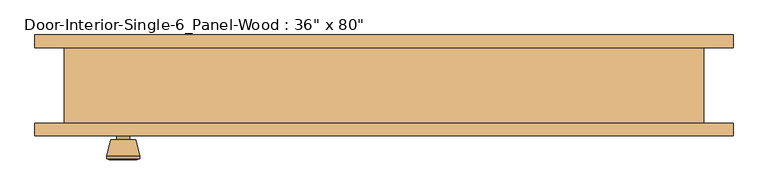
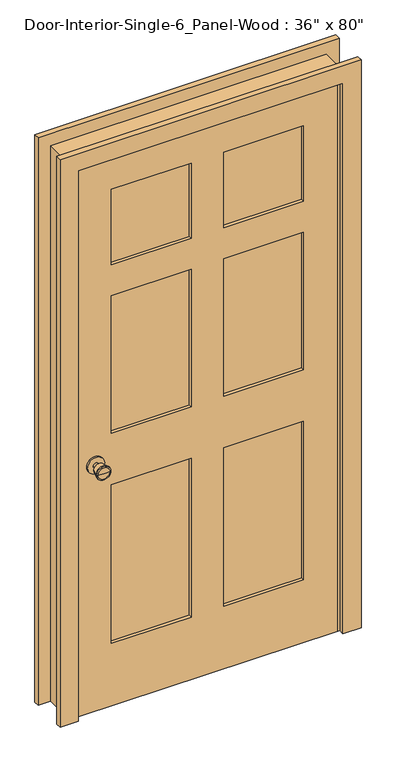
"""IFC4 building model written with IfcOpenShell, lengths in millimetres: door geometry."""

from ifc_helpers import new_model, si_unit, point, frame, frame_2d, origin, place, context, project, spatial, polyline, circle_curve, trimmed, segment, composite_curve, outline, extrude, faceted_brep, source, transform, mapped, element, save
from ifc_brep_helpers import plane_surface, cylinder_surface, revolved_surface, advanced_brep


def door_a4da38fb(model_context):
    return source(origin(), model_context, "Body", "SolidModel", [
        advanced_brep(
        [(-393.7, -13.05, 914.4), (-403.7, -13.05, 914.4), (-383.7, -13.05, 914.4), (-373.2241324, 35.95, 914.4), (-414.1758676, 35.95, 914.4), (-393.7, 35.95, 914.4), (-368.7, 34.1221319, 914.4), (-418.7, 34.1221319, 914.4), (-368.7, 30.6584537, 914.4), (-418.7, 30.6584537, 914.4), (-375.063764, 5.95, 914.4), (-412.336236, 5.95, 914.4), (-383.7, 5.95, 914.4), (-403.7, 5.95, 914.4)],
        [
            (0, 1),
            (1, 2, circle_curve(frame((-393.7, -13.05, 914.4), z_axis=(0.0, -1.0, 0.0), x_axis=(-1.0, 0.0, 0.0)), 10.0)),
            (2, 0),
            (2, 1, circle_curve(frame((-393.7, -13.05, 914.4), z_axis=(0.0, -1.0, 0.0), x_axis=(-1.0, 0.0, 0.0)), 10.0)),
            (3, 4, circle_curve(frame((-393.7, 35.95, 914.4), z_axis=(0.0, 1.0, 0.0), x_axis=(-1.0, 0.0, 0.0)), 20.4758676)),
            (4, 5),
            (5, 3),
            (4, 3, circle_curve(frame((-393.7, 35.95, 914.4), z_axis=(0.0, 1.0, 0.0), x_axis=(-1.0, 0.0, 0.0)), 20.4758676)),
            (6, 7, circle_curve(frame((-393.7, 34.1221319, 914.4), z_axis=(0.0, 1.0, 0.0), x_axis=(-1.0, 0.0, 0.0)), 25.0)),
            (7, 4),
            (3, 6),
            (7, 6, circle_curve(frame((-393.7, 34.1221319, 914.4), z_axis=(0.0, 1.0, 0.0), x_axis=(-1.0, 0.0, 0.0)), 25.0)),
            (8, 9, circle_curve(frame((-393.7, 30.6584537, 914.4), z_axis=(0.0, 1.0, 0.0), x_axis=(-1.0, 0.0, 0.0)), 25.0)),
            (9, 7),
            (6, 8),
            (9, 8, circle_curve(frame((-393.7, 30.6584537, 914.4), z_axis=(0.0, 1.0, 0.0), x_axis=(-1.0, 0.0, 0.0)), 25.0)),
            (10, 11, circle_curve(frame((-393.7, 5.95, 914.4), z_axis=(0.0, 1.0, 0.0), x_axis=(-1.0, 0.0, 0.0)), 18.636236)),
            (11, 9),
            (8, 10),
            (11, 10, circle_curve(frame((-393.7, 5.95, 914.4), z_axis=(0.0, 1.0, 0.0), x_axis=(-1.0, 0.0, 0.0)), 18.636236)),
            (12, 13, circle_curve(frame((-393.7, 5.95, 914.4), z_axis=(0.0, 1.0, 0.0), x_axis=(-1.0, 0.0, 0.0)), 10.0)),
            (13, 11),
            (10, 12),
            (13, 12, circle_curve(frame((-393.7, 5.95, 914.4), z_axis=(0.0, 1.0, 0.0), x_axis=(-1.0, 0.0, 0.0)), 10.0)),
            (1, 13),
            (12, 2),
        ],
        [
            plane_surface(frame((-393.7, -13.05, 914.4), z_axis=(0.0, -1.0, 0.0), x_axis=(-1.0, 0.0, 0.0))),
            plane_surface(frame((-393.7, 35.95, 914.4), z_axis=(0.0, 1.0, 0.0), x_axis=(-1.0, 0.0, 0.0))),
            revolved_surface(polyline([(-414.1758676, 35.95, 914.4), (-418.7, 34.1221319, 914.4)]), (-393.7, -13.05, 914.4), (0.0, -1.0, 0.0)),
            cylinder_surface(frame((-393.7, -13.05, 914.4), z_axis=(0.0, -1.0, 0.0), x_axis=(-1.0, 0.0, 0.0)), 25.0),
            revolved_surface(polyline([(-418.7, 30.6584537, 914.4), (-412.336236, 5.95, 914.4)]), (-393.7, -13.05, 914.4), (0.0, -1.0, 0.0)),
            plane_surface(frame((-393.7, 5.95, 914.4), z_axis=(0.0, -1.0, 0.0), x_axis=(-1.0, 0.0, 0.0))),
            cylinder_surface(frame((-393.7, -13.05, 914.4), z_axis=(0.0, -1.0, 0.0), x_axis=(-1.0, 0.0, 0.0)), 10.0),
        ],
        [
            (0, [[1, 2, 3]]),
            (0, [[-3, 4, -1]]),
            (1, [[5, 6, 7]]),
            (1, [[8, -7, -6]]),
            (2, [[9, 10, -5, 11]]),
            (2, [[12, -11, -8, -10]]),
            (3, [[13, 14, -9, 15]]),
            (3, [[16, -15, -12, -14]]),
            (4, [[17, 18, -13, 19]]),
            (4, [[20, -19, -16, -18]]),
            (5, [[21, 22, -17, 23]]),
            (5, [[24, -23, -20, -22]]),
            (6, [[-2, 25, -21, 26]]),
            (6, [[-4, -26, -24, -25]]),
        ],
    ),
        extrude(outline(composite_curve([segment(trimmed(circle_curve(frame_2d((914.4, -393.7)), 30.0), [point((914.4, -423.7))], [point((914.4, -363.7))], False, "CARTESIAN"), True, "CONTINUOUS"), segment(trimmed(circle_curve(frame_2d((914.4, -393.7)), 30.0), [point((914.4, -363.7))], [point((914.4, -423.7))], False, "CARTESIAN"), True, "CONTINUOUS")], self_intersect=False)), frame((0.0, -19.05, 0.0), z_axis=(0.0, 1.0, 0.0), x_axis=(0.0, 0.0, 1.0)), (0.0, 0.0, 1.0), 6.0),
        advanced_brep(
        [(-393.7, -59.975, 914.4), (-383.7, -59.975, 914.4), (-403.7, -59.975, 914.4), (-373.2241324, -108.975, 914.4), (-393.7, -108.975, 914.4), (-414.1758676, -108.975, 914.4), (-368.7, -107.1471319, 914.4), (-418.7, -107.1471319, 914.4), (-368.7, -103.6834537, 914.4), (-418.7, -103.6834537, 914.4), (-375.063764, -78.975, 914.4), (-412.336236, -78.975, 914.4), (-383.7, -78.975, 914.4), (-403.7, -78.975, 914.4)],
        [
            (0, 1),
            (1, 2, circle_curve(frame((-393.7, -59.975, 914.4), z_axis=(0.0, 1.0, 0.0), x_axis=(-1.0, 0.0, 0.0)), 10.0)),
            (2, 0),
            (2, 1, circle_curve(frame((-393.7, -59.975, 914.4), z_axis=(0.0, 1.0, 0.0), x_axis=(-1.0, 0.0, 0.0)), 10.0)),
            (3, 4),
            (4, 5),
            (5, 3, circle_curve(frame((-393.7, -108.975, 914.4), z_axis=(0.0, -1.0, 0.0), x_axis=(-1.0, 0.0, 0.0)), 20.4758676)),
            (3, 5, circle_curve(frame((-393.7, -108.975, 914.4), z_axis=(0.0, -1.0, 0.0), x_axis=(-1.0, 0.0, 0.0)), 20.4758676)),
            (6, 3),
            (5, 7),
            (7, 6, circle_curve(frame((-393.7, -107.1471319, 914.4), z_axis=(0.0, -1.0, 0.0), x_axis=(-1.0, 0.0, 0.0)), 25.0)),
            (6, 7, circle_curve(frame((-393.7, -107.1471319, 914.4), z_axis=(0.0, -1.0, 0.0), x_axis=(-1.0, 0.0, 0.0)), 25.0)),
            (8, 6),
            (7, 9),
            (9, 8, circle_curve(frame((-393.7, -103.6834537, 914.4), z_axis=(0.0, -1.0, 0.0), x_axis=(-1.0, 0.0, 0.0)), 25.0)),
            (8, 9, circle_curve(frame((-393.7, -103.6834537, 914.4), z_axis=(0.0, -1.0, 0.0), x_axis=(-1.0, 0.0, 0.0)), 25.0)),
            (10, 8),
            (9, 11),
            (11, 10, circle_curve(frame((-393.7, -78.975, 914.4), z_axis=(0.0, -1.0, 0.0), x_axis=(-1.0, 0.0, 0.0)), 18.636236)),
            (10, 11, circle_curve(frame((-393.7, -78.975, 914.4), z_axis=(0.0, -1.0, 0.0), x_axis=(-1.0, 0.0, 0.0)), 18.636236)),
            (12, 10),
            (11, 13),
            (13, 12, circle_curve(frame((-393.7, -78.975, 914.4), z_axis=(0.0, -1.0, 0.0), x_axis=(-1.0, 0.0, 0.0)), 10.0)),
            (12, 13, circle_curve(frame((-393.7, -78.975, 914.4), z_axis=(0.0, -1.0, 0.0), x_axis=(-1.0, 0.0, 0.0)), 10.0)),
            (1, 12),
            (13, 2),
        ],
        [
            plane_surface(frame((-393.7, -59.975, 914.4), z_axis=(0.0, 1.0, 0.0), x_axis=(-1.0, 0.0, 0.0))),
            plane_surface(frame((-393.7, -108.975, 914.4), z_axis=(0.0, -1.0, 0.0), x_axis=(-1.0, 0.0, 0.0))),
            revolved_surface(polyline([(-414.1758676, -108.975, 914.4), (-418.7, -107.1471319, 914.4)]), (-393.7, -59.975, 914.4), (0.0, 1.0, 0.0)),
            cylinder_surface(frame((-393.7, -59.975, 914.4), z_axis=(0.0, 1.0, 0.0), x_axis=(-1.0, 0.0, 0.0)), 25.0),
            revolved_surface(polyline([(-418.7, -103.6834537, 914.4), (-412.336236, -78.975, 914.4)]), (-393.7, -59.975, 914.4), (0.0, 1.0, 0.0)),
            plane_surface(frame((-393.7, -78.975, 914.4), z_axis=(0.0, 1.0, 0.0), x_axis=(-1.0, 0.0, 0.0))),
            cylinder_surface(frame((-393.7, -59.975, 914.4), z_axis=(0.0, 1.0, 0.0), x_axis=(-1.0, 0.0, 0.0)), 10.0),
        ],
        [
            (0, [[1, 2, 3]]),
            (0, [[-3, 4, -1]]),
            (1, [[5, 6, 7]]),
            (1, [[-6, -5, 8]]),
            (2, [[9, -7, 10, 11]]),
            (2, [[-10, -8, -9, 12]]),
            (3, [[13, -11, 14, 15]]),
            (3, [[-14, -12, -13, 16]]),
            (4, [[17, -15, 18, 19]]),
            (4, [[-18, -16, -17, 20]]),
            (5, [[21, -19, 22, 23]]),
            (5, [[-22, -20, -21, 24]]),
            (6, [[25, -23, 26, -2]]),
            (6, [[-26, -24, -25, -4]]),
        ],
    ),
        extrude(outline(composite_curve([segment(trimmed(circle_curve(frame_2d((914.4, -393.7)), 30.0), [point((914.4, -423.7))], [point((914.4, -363.7))], False, "CARTESIAN"), True, "CONTINUOUS"), segment(trimmed(circle_curve(frame_2d((914.4, -393.7)), 30.0), [point((914.4, -363.7))], [point((914.4, -423.7))], False, "CARTESIAN"), True, "CONTINUOUS")], self_intersect=False)), frame((0.0, -59.975, 0.0), z_axis=(0.0, 1.0, 0.0), x_axis=(0.0, 0.0, 1.0)), (0.0, 0.0, 1.0), 6.0),
        faceted_brep([(482.6, -53.975, 0.0), (457.2, -53.975, 0.0), (457.2, -19.05, 0.0), (444.5, -19.05, 0.0), (444.5, 15.875, 0.0), (457.2, 15.875, 0.0), (457.2, 60.325, 0.0), (482.6, 60.325, 0.0), (482.6, 60.325, 2057.4), (482.6, -53.975, 2057.4), (457.2, 60.325, 2032.0), (-457.2, 60.325, 2032.0), (-457.2, 60.325, 0.0), (-482.6, 60.325, 0.0), (-482.6, 60.325, 2057.4), (457.2, 15.875, 2032.0), (444.5, 15.875, 2019.3), (-444.5, 15.875, 2019.3), (-444.5, 15.875, 0.0), (-457.2, 15.875, 0.0), (-457.2, 15.875, 2032.0), (444.5, -19.05, 2019.3), (457.2, -19.05, 2032.0), (-457.2, -19.05, 2032.0), (-457.2, -19.05, 0.0), (-444.5, -19.05, 0.0), (-444.5, -19.05, 2019.3), (457.2, -53.975, 2032.0), (-482.6, -53.975, 2057.4), (-482.6, -53.975, 0.0), (-457.2, -53.975, 0.0), (-457.2, -53.975, 2032.0)], [[[0, 1, 2, 3, 4, 5, 6, 7]], [[7, 8, 9, 0]], [[6, 10, 11, 12, 13, 14, 8, 7]], [[5, 15, 10, 6]], [[4, 16, 17, 18, 19, 20, 15, 5]], [[3, 21, 16, 4]], [[2, 22, 23, 24, 25, 26, 21, 3]], [[1, 27, 22, 2]], [[0, 9, 28, 29, 30, 31, 27, 1]], [[8, 14, 28, 9]], [[15, 20, 11, 10]], [[21, 26, 17, 16]], [[27, 31, 23, 22]], [[29, 13, 12, 19, 18, 25, 24, 30]], [[14, 13, 29, 28]], [[20, 19, 12, 11]], [[26, 25, 18, 17]], [[31, 30, 24, 23]]]),
        extrude(outline(polyline([(2032.0, -457.2), (0.0, -457.2), (0.0, 457.2), (2032.0, 457.2), (2032.0, -457.2)]), holes=[polyline([(1912.9375, 57.15), (1912.9375, 336.55), (1633.5375, 336.55), (1633.5375, 57.15), (1912.9375, 57.15)]), polyline([(1519.2375, 336.55), (1009.65, 336.55), (1009.65, 57.15), (1519.2375, 57.15), (1519.2375, 336.55)]), polyline([(1009.65, -57.15), (1009.65, -336.55), (1519.2375, -336.55), (1519.2375, -57.15), (1009.65, -57.15)]), polyline([(1633.5375, -336.55), (1912.9375, -336.55), (1912.9375, -57.15), (1633.5375, -57.15), (1633.5375, -336.55)]), polyline([(819.15, 57.15), (819.15, 336.55), (231.775, 336.55), (231.775, 57.15), (819.15, 57.15)]), polyline([(231.775, -57.15), (231.775, -336.55), (819.15, -336.55), (819.15, -57.15), (231.775, -57.15)])]), frame((0.0, -53.975, 0.0), z_axis=(0.0, 1.0, 0.0), x_axis=(0.0, 0.0, 1.0)), (0.0, 0.0, 1.0), 34.925),
        extrude(outline(polyline([(336.55, -30.6916667), (336.55, -42.3333333), (57.15, -42.3333333), (57.15, -30.6916667), (336.55, -30.6916667)])), frame((0.0, 0.0, 1633.5375), z_axis=(0.0, 0.0, 1.0), x_axis=(1.0, 0.0, 0.0)), (0.0, 0.0, 1.0), 279.4),
        extrude(outline(polyline([(336.55, -30.6916667), (336.55, -42.3333333), (57.15, -42.3333333), (57.15, -30.6916667), (336.55, -30.6916667)])), frame((0.0, 0.0, 1009.65), z_axis=(0.0, 0.0, 1.0), x_axis=(1.0, 0.0, 0.0)), (0.0, 0.0, 1.0), 509.5875),
        extrude(outline(polyline([(-57.15, -30.6916667), (-57.15, -42.3333333), (-336.55, -42.3333333), (-336.55, -30.6916667), (-57.15, -30.6916667)])), frame((0.0, 0.0, 1009.65), z_axis=(0.0, 0.0, 1.0), x_axis=(1.0, 0.0, 0.0)), (0.0, 0.0, 1.0), 509.5875),
        extrude(outline(polyline([(-57.15, -30.6916667), (-57.15, -42.3333333), (-336.55, -42.3333333), (-336.55, -30.6916667), (-57.15, -30.6916667)])), frame((0.0, 0.0, 1633.5375), z_axis=(0.0, 0.0, 1.0), x_axis=(1.0, 0.0, 0.0)), (0.0, 0.0, 1.0), 279.4),
        extrude(outline(polyline([(336.55, -30.6916667), (336.55, -42.3333333), (57.15, -42.3333333), (57.15, -30.6916667), (336.55, -30.6916667)])), frame((0.0, 0.0, 231.775), z_axis=(0.0, 0.0, 1.0), x_axis=(1.0, 0.0, 0.0)), (0.0, 0.0, 1.0), 587.375),
        extrude(outline(polyline([(-57.15, -30.6916667), (-57.15, -42.3333333), (-336.55, -42.3333333), (-336.55, -30.6916667), (-57.15, -30.6916667)])), frame((0.0, 0.0, 231.775), z_axis=(0.0, 0.0, 1.0), x_axis=(1.0, 0.0, 0.0)), (0.0, 0.0, 1.0), 587.375),
        extrude(outline(polyline([(0.0, 527.05), (2101.85, 527.05), (2101.85, -527.05), (0.0, -527.05), (0.0, -463.55), (2038.35, -463.55), (2038.35, 463.55), (0.0, 463.55), (0.0, 527.05)])), frame((0.0, -73.025, 0.0), z_axis=(0.0, 1.0, 0.0), x_axis=(0.0, 0.0, 1.0)), (0.0, 0.0, 1.0), 19.05),
        extrude(outline(polyline([(0.0, 527.05), (2101.85, 527.05), (2101.85, -527.05), (0.0, -527.05), (0.0, -463.55), (2038.35, -463.55), (2038.35, 463.55), (0.0, 463.55), (0.0, 527.05)])), frame((0.0, 60.325, 0.0), z_axis=(0.0, 1.0, 0.0), x_axis=(0.0, 0.0, 1.0)), (0.0, 0.0, 1.0), 19.05),
    ])


if __name__ == "__main__":
    model = new_model("IFC4")
    model_context = context("Model", 3, world=origin())
    ifc_project = project(units=[si_unit("LENGTHUNIT", "METRE", prefix="MILLI")], contexts=[model_context])
    site = spatial("IfcSite", under=ifc_project)
    building = spatial("IfcBuilding", under=site)
    placement = place(None, origin())
    door_shape = door_a4da38fb(model_context)
    element("IfcDoor", 1, ObjectType="Door-Interior-Single-6_Panel-Wood : 36\" x 80\"", at=placement, inside=building, context=model_context, shape_type="MappedRepresentation", body=[
        mapped(door_shape, transform((0.0, 0.0, 0.0), x_axis=(1.0, 0.0, 0.0), y_axis=(0.0, 1.0, 0.0), z_axis=(0.0, 0.0, 1.0))),
    ])
    save(model, "model.ifc")

# Revit data of these elements
# Type "Door-Interior-Single-6_Panel-Wood : 36\" x 80\""
#   Type Mark = "9"
#   Assembly Code = "C1020300"
#   Analytic Construction = "Wooden"
#   Top Rail = 0' - 4 11/16"
#   Top Panel = 0' - 11"
#   Thickness = 0' - 1 3/8"
#   Thermal Resistance (R) = 2.5876 (h·ft²·°F)/BTU
#   Swing Angle [instance default] = 90.00°
#   Stiles = 0' - 4 3/4"
#   Rough Width = 3' - 2"
#   Rough Height = 6' - 9"
#   Mullion = 0' - 4 1/2"
#   Lock Rail = 0' - 7 1/2"
#   Intermediate Rail = 0' - 4 1/2"
#   Height = 6' - 8"
#   Width = 3' - 0"
#   Heat Transfer Coefficient (U) = 0.3865 BTU/(h·ft²·°F)
#   Bottom Rail = 0' - 9 1/8"
#   Trim Material = Cherry
#   Panel Material = Cherry
#   Frame Material = Cherry
#   Door Handle Material = Aluminum
#   Visual Light Transmittance = 0
#   Solar Heat Gain Coefficient = 0
#   Wall Closure = (empty or 0)
#   Function = (empty or 0)
# Element 1 (IfcDoor, "Door-Interior-Single-6_Panel-Wood : 36\" x 80\"")
#   Materials on its faces: "Cherry", "Aluminum"
# Materials
#   "Cherry": class "Wood", colour RGB 226 177 128, transparency 0, Description = "Prunus Serotina", Cost = 0
#   "Aluminum": class "Metal", colour RGB 247 247 247, transparency 0, Description = "Aluminum 6061", Cost = 0
